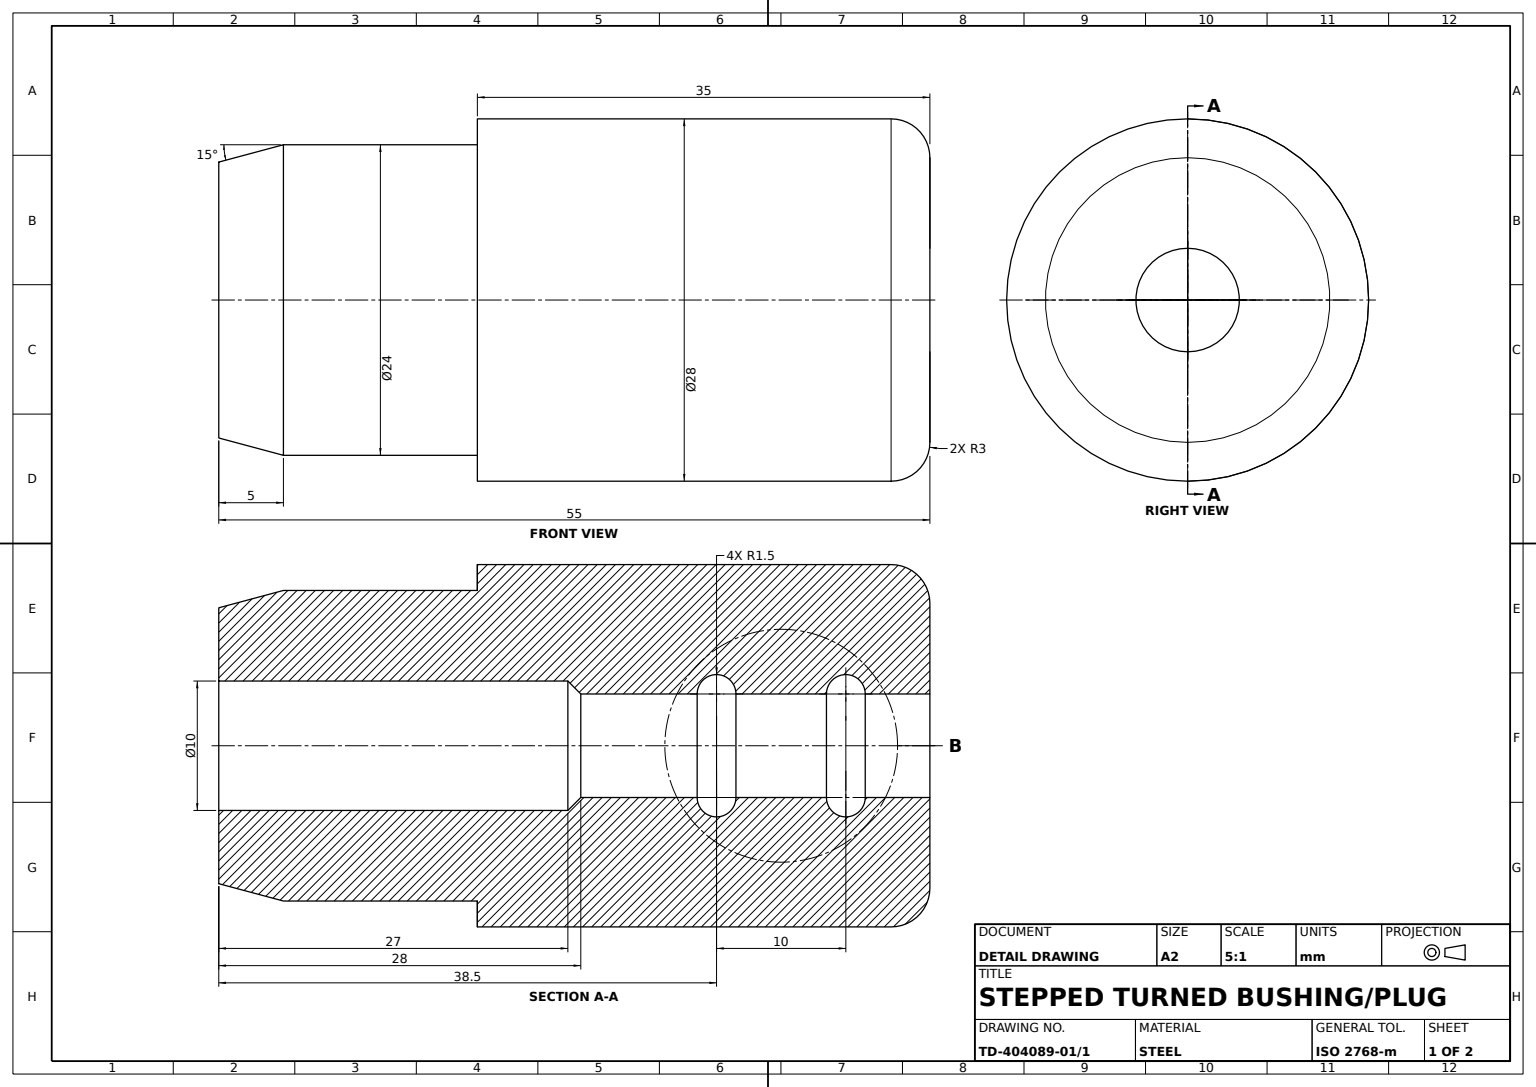
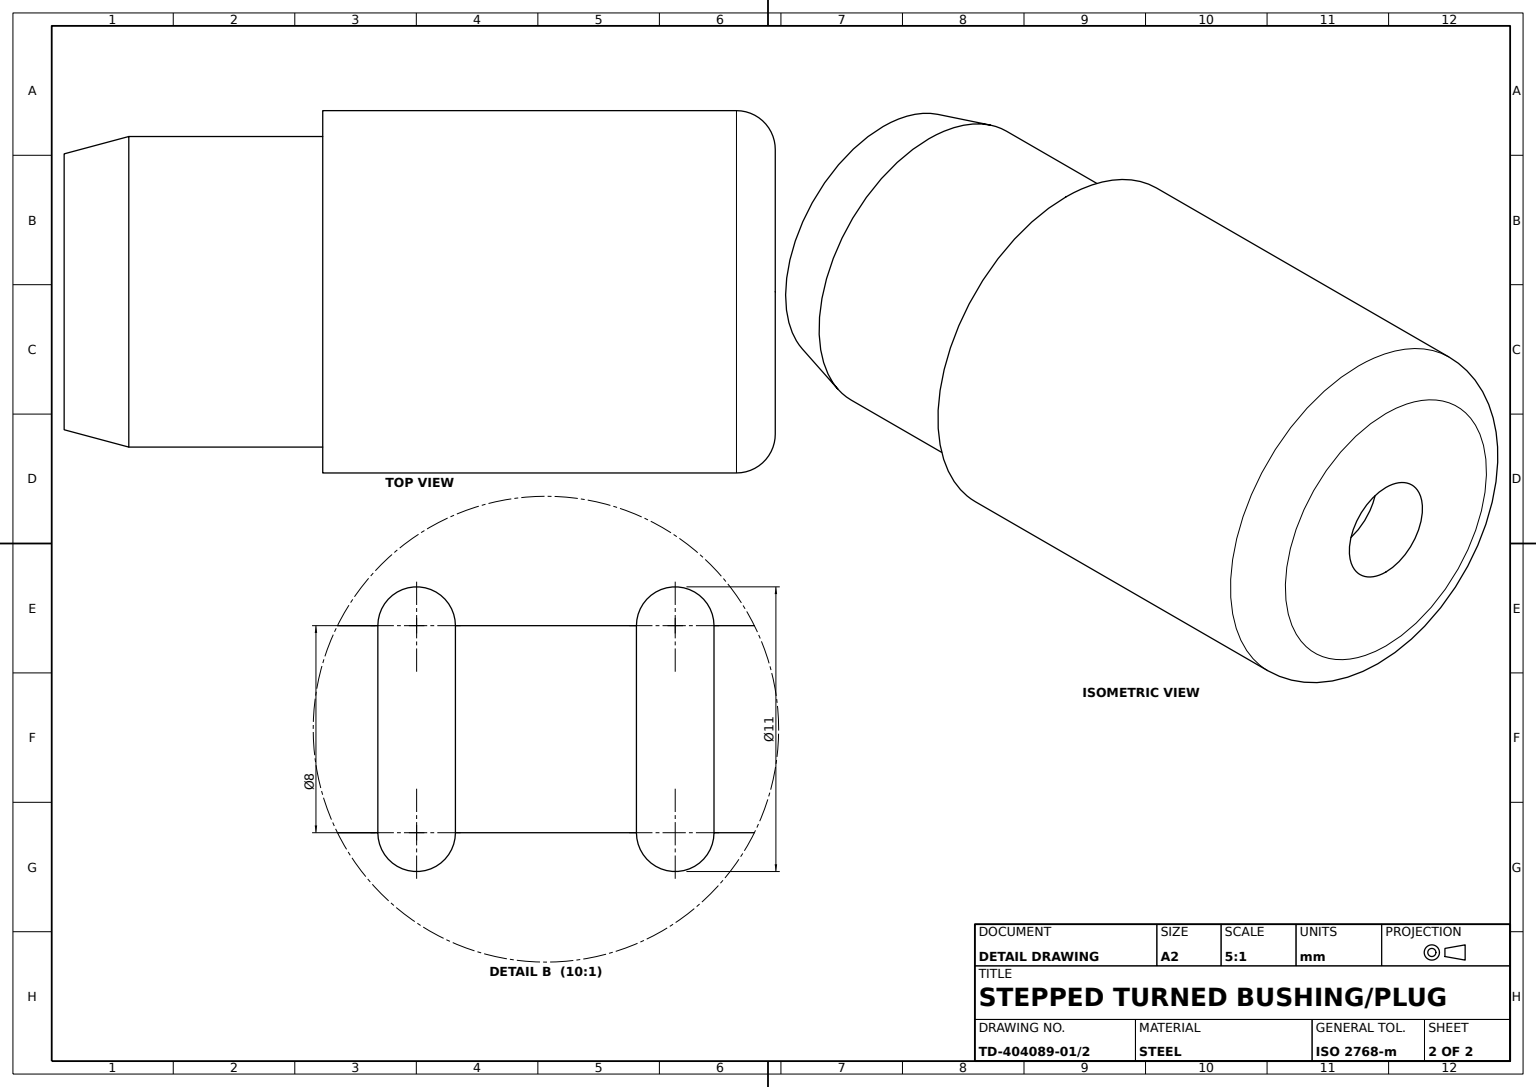
SolidWorks part; units mm, degrees
material "Plain Carbon Steel"
ref_plane "Front Plane" through (0, 0, 0) normal (0, 0, 1) x (1, 0, 0)
ref_plane "Top Plane" through (0, 0, 0) normal (0, 1, 0) x (1, 0, 0)
ref_plane "Right Plane" through (0, 0, 0) normal (1, 0, 0) x (0, 0, -1)
sketch "Pin Revolve Profile" plane through (0, 0, 0) normal (0, 0, 1) x (1, 0, 0)
  line L0 (0, 148.4515) -> (0, -93.2577) construction
  line L24 (-4, 60.1899) -> (-4, 65.1899)
  line L25 (-5, 10.1899) -> (-5, 37.1899)
  line L26 (-5, 37.1899) -> (-4, 38.1899)
  line L27 (-4, 38.1899) -> (-4, 47.1899)
  line L28 (-4, 50.1899) -> (-4, 57.1899)
  line L35 (-10.6603, 10.1899) -> (-5, 10.1899)
  line L36 (-4, 65.1899) -> (-11, 65.1899)
  line L40 (-14, 62.1899) -> (-14, 30.1899)
  line L41 (-14, 30.1899) -> (-12, 30.1899)
  line L42 (-12, 30.1899) -> (-12, 15.1899)
  line L45 (-12, 15.1899) -> (-10.6603, 10.1899)
  arc A3 (-4, 47.1899) -> (-4, 50.1899) centre (-4, 48.6899) cw
  arc A5 (-4, 57.1899) -> (-4, 60.1899) centre (-4, 58.6899) cw
  arc A6 (-11, 65.1899) -> (-14, 62.1899) centre (-11, 62.1899) ccw
  point P18 (-14, 65.1899)
  dimension "D9" = 10
  dimension "D8" = 1.5
  dimension "D7" = 3
  dimension "D6" = 1.5
  dimension "D19" = 3
  dimension "D1" = 27
  dimension "D2" = 1
  dimension "D3" = 45
  dimension "D4" = 5
  dimension "D5" = 9
  dimension "D10" = 5
  dimension "D11" = 38.1899
  dimension "D12" = 48.6899
  dimension "D13" = 58.6899
  dimension "D14" = 10
  dimension "D15" = 35
  dimension "D16" = 2
  dimension "D17" = 15
  dimension "D18" = 5
revolve "Pin Body Revolve" add sketch "Pin Revolve Profile" angle 360 about L0
